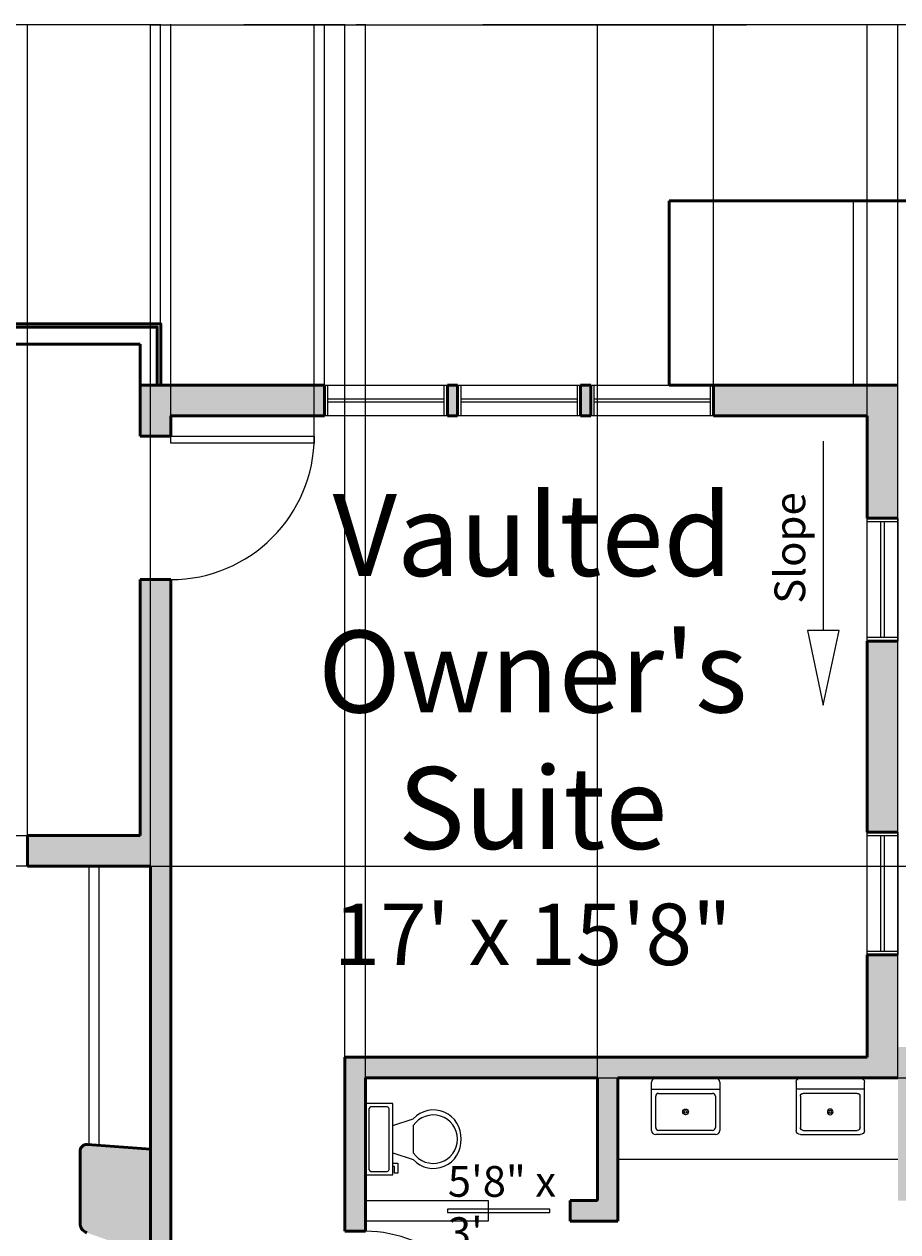
# Model space of a CAD drawing. Units: inches. Extents: x 296 to 2116, y 330 to 1460.
# Tile 5 of 9: x 752 to 1008, y 1106 to 1460. Entities that reach past the tile are written whole.
import ezdxf

# ---------------------------------------------------------------- set-up
doc = ezdxf.new("R2010")
doc.units = ezdxf.units.IN
for name, color, linetype, lineweight in [('A-ANNO-DIMS', 2, 'Continuous', 18), ('A-ANNO-SYMB', 2, 'Continuous', 18), ('A-ANNO-TEXT', 7, 'Continuous', 18), ('A-AREA-IDEN', 7, 'Continuous', 25), ('A-DOOR', 3, 'Continuous', 25), ('A-FLOR-FIXT', 8, 'Continuous', 18), ('A-FLOR-STRS', 40, 'Continuous', 25), ('A-GLAZ', 4, 'Continuous', 25), ('A-WALL', 7, 'Continuous', 50), ('A-WALL-PATT', 8, 'Continuous', 13)]:
    doc.layers.add(name, color=color, linetype=linetype, lineweight=lineweight)
doc.styles.add('ATTR', font='romans.shx', dxfattribs={"width": 0.8, "height": 1.075})
doc.styles.get("Standard").update_dxf_attribs({"font": 'arial.ttf'})
doc.dimstyles.get("Standard").update_dxf_attribs({"dimtxt": 0.18, "dimasz": 0.18, "dimexe": 0.18, "dimexo": 0.0625, "dimgap": 0.09, "dimtad": 0, "dimtih": 1, "dimtoh": 1, "dimdec": 4, "dimzin": 0, "dimdsep": 46, "dimtxsty": 'Standard', "dimcen": 0.09, "dimadec": 0, "dimazin": 0, "dimtfac": 1, "dimtdec": 4, "dimtofl": 0, "dimtmove": 0, "dimatfit": 3, "dimfxl": 1, "dimtolj": 1, "dimtzin": 0, "dimarcsym": 0})

# ---------------------------------------------------------------- blocks, each defined once
blk = doc.blocks.new('*U16')
for p, q in [((0, 0), (0, 4)), ((36, 0), (36, 4))]:
    blk.add_line(p, q)
blk.add_lwpolyline([(0, 0), (25.46, -25.46), (26.69, -24.22), (1.24, 1.24)], close=True)
blk.add_arc((0, 0), 36, 315, 0)
blk = doc.blocks.new('*U27')
for p, q in [((-36, 0), (-36, 4)), ((0, 0), (0, 4))]:
    blk.add_line(p, q)
blk.add_lwpolyline([(0, 0), (0, -36), (-1.75, -36), (-1.75, 0)], close=True)
blk.add_arc((0, 0), 36, 180, 270)
blk = doc.blocks.new('*U29')
for p, q in [((9.5, -6), (9.5, -2)), ((-10, -8.5), (-8, -8.5)), ((-10, -9.5), (-10, -8.5)), ((-7, -9.5), (-10, -9.5)), ((-8, -8.5), (-8, -8)), ((-7, -8), (-7, -9.5)), ((-4, -8), (-6, -14)), ((4, -8), (6, -14)), ((4, -14), (-4, -14))]:
    blk.add_line(p, q)
blk.add_lwpolyline([(10.5, -8), (10.5, 0), (-10.5, 0), (-10.5, -8)], close=True)
for points in [[(-9.5, -2), (-9.5, -6)], [(8.5, -1), (-8.5, -1)], [(-8.5, -7), (8.5, -7)]]:
    blk.add_lwpolyline(points)
for centre, radius, start, end in [((-8.625, -1.875), 0.8839, 81.8699, 188.1301), ((8.625, -1.875), 0.8839, 351.8699, 98.1301), ((-8.625, -6.125), 0.8839, 171.869898, 278.1301), ((8.625, -6.125), 0.8839, 261.8699, 8.1301), ((-0.4772, -19.9188), 8.0953, 133.01722, 273.38), ((0.0374, -19.8731), 7.127, 124.50543, 269.7), ((-0.0373, -19.8731), 7.127, 270.3, 55.4946), ((0.4773, -19.9188), 8.0953, 266.62, 46.9828)]:
    blk.add_arc(centre, radius, start, end)
blk = doc.blocks.new("24'' Sink Single PV")
blk.add_line((-12.00001, -3.999996), (12, -3.999996))
for points in [[(-10.5, 0), (10.5, 0)], [(-12.00001, -18.499996), (-12.00001, -1.5)], [(12, -1.5), (12, -18.499996)], [(-10.5, -17.499996), (-10.5, -6.499996)], [(-9.5, -5.499996), (9.5, -5.499996)], [(10.5, -6.499996), (10.5, -17.499996)], [(10.5, -19.999996), (-10.5, -19.999996)], [(9.5, -18.499996), (-9.5, -18.499996)]]:
    blk.add_lwpolyline(points)
for radius in [1, 0.5]:
    blk.add_circle((0, -11.999996), radius)
for centre, radius, start, end in [((-10.5, -1.5), 1.5, 90, 180), ((10.5, -1.5), 1.5, 0, 90), ((-9.5, -6.499996), 1, 90, 180), ((9.5, -6.499996), 1, 0, 90), ((-10.5, -18.499996), 1.5, 180, 270), ((-9.5, -17.499996), 1, 180, 270), ((9.5, -17.499996), 1, 270, 0), ((10.5, -18.499996), 1.5, 270, 0)]:
    blk.add_arc(centre, radius, start, end)
at = {"style": 'ATTR', "width": 0.8, "flags": 9}
blk.add_attdef('ESTCODE', (0, 0), '', height=0.0048, dxfattribs=at)
blk = doc.blocks.new('SLOPE-ARROW')
blk.add_line((739.99, 662.71), (684.54, 662.71))
blk.add_lwpolyline([(662.67, 662.71), (684.54, 658.1), (684.54, 667.32)], close=True)
blk = doc.blocks.new('*D45')
at = {"layer": 'A-ANNO-DIMS', "color": 0, "lineweight": -2, "transparency": 16777216}
for p, q in [((1156.58, 1407.95), (1235.3, 1407.95)), ((1235.12, 1407.77), (1235.12, 895.66)), ((1235.12, 383.18), (1235.12, 895.29)), ((609.63, 383), (1235.3, 383))]:
    blk.add_line(p, q, dxfattribs=at)
at = {"layer": 'A-ANNO-DIMS', "color": 0, "transparency": 16777216}
for points in [[(1235.09, 1407.77), (1235.15, 1407.77), (1235.12, 1407.95)], [(1235.09, 383.18), (1235.15, 383.18), (1235.12, 383)]]:
    blk.add_solid(points, dxfattribs=at)
at = {"layer": 'Defpoints', "color": 0, "transparency": 16777216}
for p in [(1156.52, 1407.95), (1235.12, 1407.95), (609.57, 383)]:
    blk.add_point(p, dxfattribs=at)
at = {"layer": 'A-ANNO-DIMS', "color": 0, "transparency": 16777216, "insert": (1235.12, 895.48), "char_height": 0.18, "attachment_point": 5}
blk.add_mtext('\\A1;1025', dxfattribs=at)
blk = doc.blocks.new('*D46')
at = {"layer": 'A-ANNO-DIMS', "color": 0, "lineweight": -2, "transparency": 16777216}
for p, q in [((399.52, 1371.02), (399.52, 1459.73)), ((399.7, 1459.55), (595.23, 1459.55)), ((791.34, 1459.55), (595.81, 1459.55)), ((791.52, 1372.02), (791.52, 1459.73))]:
    blk.add_line(p, q, dxfattribs=at)
at = {"layer": 'A-ANNO-DIMS', "color": 0, "transparency": 16777216}
for points in [[(399.7, 1459.58), (399.7, 1459.52), (399.52, 1459.55)], [(791.34, 1459.58), (791.34, 1459.52), (791.52, 1459.55)]]:
    blk.add_solid(points, dxfattribs=at)
at = {"layer": 'Defpoints', "color": 0, "transparency": 16777216}
for p in [(791.52, 1459.55), (399.52, 1370.95), (791.52, 1371.95)]:
    blk.add_point(p, dxfattribs=at)
at = {"layer": 'A-ANNO-DIMS', "color": 0, "transparency": 16777216, "insert": (595.52, 1459.55), "char_height": 0.18, "attachment_point": 5}
blk.add_mtext('\\A1;392', dxfattribs=at)
blk = doc.blocks.new('*D47')
at = {"layer": 'A-ANNO-DIMS', "color": 0, "lineweight": -2, "transparency": 16777216}
for p, q in [((791.52, 1372.02), (791.52, 1459.73)), ((791.7, 1459.55), (946.75, 1459.55)), ((1102.34, 1459.55), (947.29, 1459.55)), ((1102.52, 1354.02), (1102.52, 1459.73))]:
    blk.add_line(p, q, dxfattribs=at)
at = {"layer": 'A-ANNO-DIMS', "color": 0, "transparency": 16777216}
for points in [[(791.7, 1459.58), (791.7, 1459.52), (791.52, 1459.55)], [(1102.34, 1459.58), (1102.34, 1459.52), (1102.52, 1459.55)]]:
    blk.add_solid(points, dxfattribs=at)
at = {"layer": 'Defpoints', "color": 0, "transparency": 16777216}
for p in [(1102.52, 1459.55), (791.52, 1371.95), (1102.52, 1353.95)]:
    blk.add_point(p, dxfattribs=at)
at = {"layer": 'A-ANNO-DIMS', "color": 0, "transparency": 16777216, "insert": (947.02, 1459.55), "char_height": 0.18, "attachment_point": 5}
blk.add_mtext('\\A1;311', dxfattribs=at)
blk = doc.blocks.new('*D77')
at = {"layer": 'A-ANNO-DIMS', "color": 0, "lineweight": -2, "transparency": 16777216}
for p, q in [((845.52, 1157.02), (845.52, 1459.73)), ((845.7, 1459.55), (848.2, 1459.55)), ((851.34, 1459.55), (848.85, 1459.55)), ((851.52, 1151.02), (851.52, 1459.73))]:
    blk.add_line(p, q, dxfattribs=at)
at = {"layer": 'A-ANNO-DIMS', "color": 0, "transparency": 16777216}
for points in [[(845.7, 1459.58), (845.7, 1459.52), (845.52, 1459.55)], [(851.34, 1459.58), (851.34, 1459.52), (851.52, 1459.55)]]:
    blk.add_solid(points, dxfattribs=at)
at = {"layer": 'Defpoints', "color": 0, "transparency": 16777216}
for p in [(851.52, 1459.55), (845.52, 1156.95), (851.52, 1150.95)]:
    blk.add_point(p, dxfattribs=at)
at = {"layer": 'A-ANNO-DIMS', "color": 0, "transparency": 16777216, "insert": (848.52, 1459.55), "char_height": 0.18, "attachment_point": 5}
blk.add_mtext('\\A1;6.00', dxfattribs=at)
blk = doc.blocks.new('*D78')
at = {"layer": 'A-ANNO-DIMS', "color": 0, "lineweight": -2, "transparency": 16777216}
for p, q in [((398.52, 1192.06), (398.52, 1459.73)), ((398.7, 1459.55), (593.06, 1459.55)), ((788.34, 1459.55), (593.99, 1459.55)), ((788.52, 1213.06), (788.52, 1459.73))]:
    blk.add_line(p, q, dxfattribs=at)
at = {"layer": 'A-ANNO-DIMS', "color": 0, "transparency": 16777216}
for points in [[(398.7, 1459.58), (398.7, 1459.52), (398.52, 1459.55)], [(788.34, 1459.58), (788.34, 1459.52), (788.52, 1459.55)]]:
    blk.add_solid(points, dxfattribs=at)
at = {"layer": 'Defpoints', "color": 0, "transparency": 16777216}
for p in [(788.52, 1459.55), (788.52, 1213), (398.52, 1192)]:
    blk.add_point(p, dxfattribs=at)
at = {"layer": 'A-ANNO-DIMS', "color": 0, "transparency": 16777216, "insert": (593.52, 1459.55), "char_height": 0.18, "attachment_point": 5}
blk.add_mtext('\\A1;390.00', dxfattribs=at)
blk = doc.blocks.new('*D79')
at = {"layer": 'A-ANNO-DIMS', "color": 0, "lineweight": -2, "transparency": 16777216}
for p, q in [((788.522265, 1213.061588), (788.522265, 1459.734098)), ((788.702265, 1459.554098), (816.628868, 1459.554098)), ((845.342265, 1459.554098), (817.415662, 1459.554098)), ((845.522265, 1157.016598), (845.522265, 1459.734098))]:
    blk.add_line(p, q, dxfattribs=at)
at = {"layer": 'A-ANNO-DIMS', "color": 0, "transparency": 16777216}
for points in [[(788.702265, 1459.584098), (788.702265, 1459.524098), (788.522265, 1459.554098)], [(845.342265, 1459.584098), (845.342265, 1459.524098), (845.522265, 1459.554098)]]:
    blk.add_solid(points, dxfattribs=at)
at = {"layer": 'Defpoints', "color": 0, "transparency": 16777216}
for p in [(845.522265, 1459.554098), (788.522265, 1212.999088), (845.522265, 1156.954098)]:
    blk.add_point(p, dxfattribs=at)
at = {"layer": 'A-ANNO-DIMS', "color": 0, "transparency": 16777216, "insert": (817.022265, 1459.554098), "char_height": 0.18, "attachment_point": 5}
blk.add_mtext('\\A1;57.00', dxfattribs=at)
blk = doc.blocks.new('*D80')
at = {"layer": 'A-ANNO-DIMS', "color": 0, "lineweight": -2, "transparency": 16777216}
for p, q in [((851.52, 1151.02), (851.52, 1459.73)), ((851.7, 1459.55), (885.13, 1459.55)), ((919.34, 1459.55), (885.92, 1459.55)), ((919.52, 1115.02), (919.52, 1459.73))]:
    blk.add_line(p, q, dxfattribs=at)
at = {"layer": 'A-ANNO-DIMS', "color": 0, "transparency": 16777216}
for points in [[(851.7, 1459.58), (851.7, 1459.52), (851.52, 1459.55)], [(919.34, 1459.58), (919.34, 1459.52), (919.52, 1459.55)]]:
    blk.add_solid(points, dxfattribs=at)
at = {"layer": 'Defpoints', "color": 0, "transparency": 16777216}
for p in [(919.52, 1459.55), (851.52, 1150.95), (919.52, 1114.95)]:
    blk.add_point(p, dxfattribs=at)
at = {"layer": 'A-ANNO-DIMS', "color": 0, "transparency": 16777216, "insert": (885.52, 1459.55), "char_height": 0.18, "attachment_point": 5}
blk.add_mtext('\\A1;68.00', dxfattribs=at)
blk = doc.blocks.new('*D81')
at = {"layer": 'A-ANNO-DIMS', "color": 0, "lineweight": -2, "transparency": 16777216}
for p, q in [((919.52, 1115.02), (919.52, 1459.73)), ((919.7, 1459.55), (963.13, 1459.55)), ((1007.34, 1459.55), (963.92, 1459.55)), ((1007.52, 1151.02), (1007.52, 1459.73))]:
    blk.add_line(p, q, dxfattribs=at)
at = {"layer": 'A-ANNO-DIMS', "color": 0, "transparency": 16777216}
for points in [[(919.7, 1459.58), (919.7, 1459.52), (919.52, 1459.55)], [(1007.34, 1459.58), (1007.34, 1459.52), (1007.52, 1459.55)]]:
    blk.add_solid(points, dxfattribs=at)
at = {"layer": 'Defpoints', "color": 0, "transparency": 16777216}
for p in [(1007.52, 1459.55), (1007.52, 1150.95), (919.52, 1114.95)]:
    blk.add_point(p, dxfattribs=at)
at = {"layer": 'A-ANNO-DIMS', "color": 0, "transparency": 16777216, "insert": (963.52, 1459.55), "char_height": 0.18, "attachment_point": 5}
blk.add_mtext('\\A1;88.00', dxfattribs=at)
blk = doc.blocks.new('*D82')
at = {"layer": 'A-ANNO-DIMS', "color": 0, "lineweight": -2, "transparency": 16777216}
for p, q in [((794.52, 1345.02), (794.52, 1459.73)), ((794.7, 1459.55), (896.06, 1459.55)), ((998.34, 1459.55), (896.99, 1459.55)), ((998.52, 1345.02), (998.52, 1459.73))]:
    blk.add_line(p, q, dxfattribs=at)
at = {"layer": 'A-ANNO-DIMS', "color": 0, "transparency": 16777216}
for points in [[(794.7, 1459.58), (794.7, 1459.52), (794.52, 1459.55)], [(998.34, 1459.58), (998.34, 1459.52), (998.52, 1459.55)]]:
    blk.add_solid(points, dxfattribs=at)
at = {"layer": 'Defpoints', "color": 0, "transparency": 16777216}
for p in [(998.52, 1459.55), (794.52, 1344.95), (998.52, 1344.95)]:
    blk.add_point(p, dxfattribs=at)
at = {"layer": 'A-ANNO-DIMS', "color": 0, "transparency": 16777216, "insert": (896.52, 1459.55), "char_height": 0.18, "attachment_point": 5}
blk.add_mtext('\\A1;204.00', dxfattribs=at)
blk = doc.blocks.new('*D83')
at = {"layer": 'A-ANNO-DIMS', "color": 0, "lineweight": -2, "transparency": 16777216}
for p, q in [((851.58, 1150.95), (1235.3, 1150.95)), ((1235.12, 1150.77), (1235.12, 1109.14)), ((1235.12, 1067.13), (1235.12, 1108.77)), ((851.58, 1066.95), (1235.3, 1066.95))]:
    blk.add_line(p, q, dxfattribs=at)
at = {"layer": 'A-ANNO-DIMS', "color": 0, "transparency": 16777216}
for points in [[(1235.09, 1150.77), (1235.15, 1150.77), (1235.12, 1150.95)], [(1235.09, 1067.13), (1235.15, 1067.13), (1235.12, 1066.95)]]:
    blk.add_solid(points, dxfattribs=at)
at = {"layer": 'Defpoints', "color": 0, "transparency": 16777216}
for p in [(851.52, 1150.95), (1235.12, 1150.95), (851.52, 1066.95)]:
    blk.add_point(p, dxfattribs=at)
at = {"layer": 'A-ANNO-DIMS', "color": 0, "transparency": 16777216, "insert": (1235.12, 1108.95), "char_height": 0.18, "attachment_point": 5}
blk.add_mtext('\\A1;84.00', dxfattribs=at)
blk = doc.blocks.new('*D85')
at = {"layer": 'A-ANNO-DIMS', "color": 0, "lineweight": -2, "transparency": 16777216}
for p, q in [((788.58, 1213), (1235.3, 1213)), ((1235.12, 1212.82), (1235.12, 1075.18)), ((1235.12, 937.18), (1235.12, 1074.82)), ((788.58, 937), (1235.3, 937))]:
    blk.add_line(p, q, dxfattribs=at)
at = {"layer": 'A-ANNO-DIMS', "color": 0, "transparency": 16777216}
for points in [[(1235.09, 1212.82), (1235.15, 1212.82), (1235.12, 1213)], [(1235.09, 937.18), (1235.15, 937.18), (1235.12, 937)]]:
    blk.add_solid(points, dxfattribs=at)
at = {"layer": 'Defpoints', "color": 0, "transparency": 16777216}
for p in [(788.52, 1213), (1235.12, 1213), (788.52, 937)]:
    blk.add_point(p, dxfattribs=at)
at = {"layer": 'A-ANNO-DIMS', "color": 0, "transparency": 16777216, "insert": (1235.12, 1075), "char_height": 0.18, "attachment_point": 5}
blk.add_mtext('\\A1;276.00', dxfattribs=at)
blk = doc.blocks.new('*D100')
at = {"layer": 'A-ANNO-DIMS', "color": 0, "lineweight": -2, "transparency": 16777216}
for p, q in [((794.52, 1339.02), (794.52, 1459.73)), ((794.7, 1459.55), (815.13, 1459.55)), ((836.34, 1459.55), (815.92, 1459.55)), ((836.52, 1339.02), (836.52, 1459.73))]:
    blk.add_line(p, q, dxfattribs=at)
at = {"layer": 'A-ANNO-DIMS', "color": 0, "transparency": 16777216}
for points in [[(794.7, 1459.58), (794.7, 1459.52), (794.52, 1459.55)], [(836.34, 1459.58), (836.34, 1459.52), (836.52, 1459.55)]]:
    blk.add_solid(points, dxfattribs=at)
at = {"layer": 'Defpoints', "color": 0, "transparency": 16777216}
for p in [(836.52, 1459.55), (794.52, 1338.95), (836.52, 1338.95)]:
    blk.add_point(p, dxfattribs=at)
at = {"layer": 'A-ANNO-DIMS', "color": 0, "transparency": 16777216, "insert": (815.52, 1459.55), "char_height": 0.18, "attachment_point": 5}
blk.add_mtext('\\A1;42.00', dxfattribs=at)
blk = doc.blocks.new('*D104')
at = {"layer": 'A-ANNO-DIMS', "color": 0, "lineweight": -2, "transparency": 16777216}
for p, q in [((612.52, 1222.06), (612.52, 1459.73)), ((612.7, 1459.55), (682.07, 1459.55)), ((752.34, 1459.55), (682.98, 1459.55)), ((752.52, 1222.06), (752.52, 1459.73))]:
    blk.add_line(p, q, dxfattribs=at)
at = {"layer": 'A-ANNO-DIMS', "color": 0, "transparency": 16777216}
for points in [[(612.7, 1459.58), (612.7, 1459.52), (612.52, 1459.55)], [(752.34, 1459.58), (752.34, 1459.52), (752.52, 1459.55)]]:
    blk.add_solid(points, dxfattribs=at)
at = {"layer": 'Defpoints', "color": 0, "transparency": 16777216}
for p in [(752.52, 1459.55), (612.52, 1222), (752.52, 1222)]:
    blk.add_point(p, dxfattribs=at)
at = {"layer": 'A-ANNO-DIMS', "color": 0, "transparency": 16777216, "insert": (682.52, 1459.55), "char_height": 0.18, "attachment_point": 5}
blk.add_mtext('\\A1;140.00', dxfattribs=at)
blk = doc.blocks.new('*D106')
at = {"layer": 'A-ANNO-DIMS', "color": 0, "lineweight": -2, "transparency": 16777216}
for p, q in [((839.52, 1354.02), (839.52, 1459.73)), ((839.7, 1459.55), (896.07, 1459.55)), ((953.34, 1459.55), (896.98, 1459.55)), ((953.52, 1354.02), (953.52, 1459.73))]:
    blk.add_line(p, q, dxfattribs=at)
at = {"layer": 'A-ANNO-DIMS', "color": 0, "transparency": 16777216}
for points in [[(839.7, 1459.58), (839.7, 1459.52), (839.52, 1459.55)], [(953.34, 1459.58), (953.34, 1459.52), (953.52, 1459.55)]]:
    blk.add_solid(points, dxfattribs=at)
at = {"layer": 'Defpoints', "color": 0, "transparency": 16777216}
for p in [(953.52, 1459.55), (839.52, 1353.95), (953.52, 1353.95)]:
    blk.add_point(p, dxfattribs=at)
at = {"layer": 'A-ANNO-DIMS', "color": 0, "transparency": 16777216, "insert": (896.52, 1459.55), "char_height": 0.18, "attachment_point": 5}
blk.add_mtext('\\A1;114.00', dxfattribs=at)

msp = doc.modelspace()

# ---------------------------------------------------------------- hatches: boundary and pattern name
at = {"layer": 'A-WALL-PATT'}
h = msp.add_hatch(color=256, dxfattribs=at)
h.dxf.hatch_style = 1
h.paths.add_polyline_path([(656.5723, 927.9991), (668.5723, 927.9991), (668.5723, 936.9991), (650.5723, 936.9991), (650.5723, 897.9991), (356.5223, 897.9991), (356.5223, 955.9991), (347.5223, 955.9991), (347.5223, 888.9991), (423.5723, 888.9991), (423.5723, 766.9991), (432.5723, 766.9991), (432.5723, 834.9991), (453.5723, 834.9991), (468.5723, 834.9991), (468.5723, 840.9991), (432.5723, 840.9991), (432.5723, 888.9991), (504.5723, 888.9991), (504.5723, 840.9991), (504.5723, 834.9991), (531.6223, 834.9991), (531.6223, 768.5344), (527.8443, 764.7564), (530.6728, 761.928), (532.087, 760.5138), (540.5723, 768.9991), (598.0723, 768.9991), (598.0723, 777.9991), (601.8223, 777.9991), (601.8223, 782.1991), (601.8223, 783.9991), (598.0723, 783.9991), (598.0723, 798.9991), (592.0723, 798.9991), (592.0723, 774.9991), (537.6223, 774.9991), (537.6223, 834.9991), (592.0723, 834.9991), (592.0723, 828.9991), (598.0723, 828.9991), (598.0723, 834.9991), (647.5723, 834.9991), (647.5723, 828.9991), (656.5723, 828.9991), (656.5723, 846.9991), (650.5723, 846.9991), (647.5723, 846.9991), (647.5723, 840.9991), (510.5723, 840.9991), (510.5723, 888.9991), (647.5723, 888.9991), (647.5723, 882.9991), (656.5723, 882.9991)])
h.paths.add_polyline_path([(432.5723, 730.9991), (496.5723, 730.9991), (496.5723, 724.9991), (502.5723, 724.9991), (502.5723, 730.9991), (506.6311, 735.058), (502.3885, 739.3006), (500.087, 736.9991), (432.5723, 736.9991), (432.5723, 742.9991), (423.5723, 742.9991), (423.5723, 641.9991), (490.5723, 641.9991), (490.5723, 597.9991), (531.5723, 597.9991), (531.5723, 606.9991), (499.5723, 606.9991), (499.5723, 650.9991), (502.5723, 650.9991), (502.5723, 659.9991), (496.5723, 659.9991), (493.5723, 659.9991), (493.5723, 650.9991), (432.5723, 650.9991)])
h.paths.add_polyline_path([(656.5723, 689.4991), (662.5473, 689.4991), (662.5473, 698.4991), (656.5723, 698.4991), (656.5723, 789.9991), (647.5723, 789.9991), (647.5723, 783.9991), (643.8223, 783.9991), (643.8223, 777.9991), (647.5723, 777.9991), (647.5723, 606.9991), (615.5723, 606.9991), (615.5723, 597.9991), (656.5723, 597.9991)])
h.paths.add_polyline_path([(761.5223, 780.9541), (797.5223, 780.9541), (797.5223, 789.9541), (761.5223, 789.9541), (761.5223, 858.9541), (797.5223, 858.9541), (797.5223, 867.9541), (752.5223, 867.9541), (752.5223, 698.4991), (746.5473, 698.4991), (746.5473, 694.2991), (746.5473, 689.4991), (752.5223, 689.4991), (752.5223, 624.9541), (761.5223, 624.9541)])
h.paths.add_polyline_path([(1102.5223, 795.9541), (1093.5223, 795.9541), (1093.5223, 789.9541), (1063.5223, 789.9541), (881.5223, 789.9541), (881.5223, 837.9541), (911.5223, 837.9541), (911.5223, 849.9541), (907.5223, 849.9541), (905.5223, 849.9541), (905.5223, 843.9541), (845.5223, 843.9541), (845.5223, 834.9541), (849.0223, 834.9541), (851.5223, 834.9541), (851.5223, 837.9541), (875.5223, 837.9541), (875.5223, 789.9541), (851.5223, 789.9541), (851.5223, 792.9541), (845.5223, 792.9541), (845.5223, 789.9541), (833.5223, 789.9541), (833.5223, 785.1541), (833.5223, 780.9541), (1049.5223, 780.9541), (1049.5223, 726.9541), (1053.7223, 726.9541), (1058.5223, 726.9541), (1058.5223, 780.9541), (1102.5223, 780.9541)])
h.paths.add_polyline_path([(761.5223, 588.9541), (752.5223, 588.9541), (752.5223, 564.9541), (761.5223, 564.9541)])
h.paths.add_polyline_path([(809.5223, 480.9541), (761.5223, 480.9541), (761.5223, 528.9541), (752.5223, 528.9541), (752.5223, 471.9541), (809.5223, 471.9541)])
h.paths.add_polyline_path([(1058.5223, 684.9541), (1049.5223, 684.9541), (1049.5223, 480.9541), (1001.5223, 480.9541), (1001.5223, 476.4541), (1001.5223, 471.9541), (1058.5223, 471.9541)])
h.paths.add_polyline_path([(794.5223, 1013.9991), (800.5223, 1013.9991), (800.5223, 1019.9991), (794.5223, 1019.9991), (794.5223, 1296.9541), (785.5223, 1296.9541), (785.5223, 1221.9991), (752.5223, 1221.9991), (752.5223, 1212.9991), (788.5223, 1212.9991), (788.5223, 936.9991), (752.5223, 936.9991), (752.5223, 927.9991), (794.5223, 927.9991)])
h.paths.add_polyline_path([(450.0223, 1191.9991), (398.5223, 1191.9991), (398.5223, 1137.9991), (407.5223, 1137.9991), (407.5223, 1182.9991), (450.0223, 1182.9991)])
h.paths.add_polyline_path([(576.5223, 1212.9991), (612.5223, 1212.9991), (612.5223, 1221.9991), (567.5223, 1221.9991), (567.5223, 1191.9991), (540.0223, 1191.9991), (540.0223, 1182.9991), (576.5223, 1182.9991)])
h.paths.add_polyline_path([(407.5223, 1060.9991), (398.5223, 1060.9991), (398.5223, 1030.9991), (392.5223, 1030.9991), (392.5223, 1021.9991), (407.5223, 1021.9991)])
h.paths.add_polyline_path([(356.5223, 1030.9991), (347.5223, 1030.9991), (347.5223, 1015.9991), (356.5223, 1015.9991), (356.5223, 1021.9991)])
h.paths.add_polyline_path([(788.5223, 1129.9991), (770.0334, 1131.3572, 0.43585667), (767.8869, 1129.3626), (767.8869, 1108.3618, 0.31855172), (769.8942, 1105.5308), (788.5223, 1098.9991)], flags=17)
h.paths.add_polyline_path([(788.5223, 1050.9991), (769.8942, 1044.4674, 0.31855172), (767.8869, 1041.6364), (767.8869, 1020.6356, 0.43585667), (770.0334, 1018.641), (788.5223, 1019.9991)], flags=17)
h.paths.add_polyline_path([(893.5223, 1066.9541), (851.5223, 1066.9541), (851.5223, 1069.9541), (845.5223, 1069.9541), (845.5223, 1019.9991), (839.5223, 1019.9991), (839.5223, 1013.9991), (845.5223, 1013.9991), (845.5223, 891.9541), (863.5223, 891.9541), (863.5223, 897.9541), (851.5223, 897.9541), (851.5223, 927.9541), (905.5223, 927.9541), (905.5223, 897.9541), (893.5223, 897.9541), (893.5223, 891.9541), (905.5223, 891.9541), (905.5223, 885.9541), (911.5223, 885.9541), (911.5223, 927.9541), (1030.5223, 927.9541), (1030.5223, 936.9541), (1013.5223, 936.9541), (1013.5223, 996.9541), (1093.5223, 996.9541), (1093.5223, 936.9541), (1066.5223, 936.9541), (1066.5223, 927.9541), (1093.5223, 927.9541), (1093.5223, 921.9541), (1102.5223, 921.9541), (1102.5223, 1013.9541), (1093.5223, 1013.9541), (1093.5223, 1002.9541), (1013.5223, 1002.9541), (1013.5223, 1060.9541), (1013.5223, 1066.9541), (1007.5223, 1066.9541), (1007.5223, 1042.9541), (977.5223, 1042.9541), (977.5223, 1066.9541), (965.5223, 1066.9541), (965.5223, 1060.9541), (971.5223, 1060.9541), (971.5223, 1036.9541), (1007.5223, 1036.9541), (1007.5223, 936.9541), (851.5223, 936.9541), (851.5223, 1060.9541), (893.5223, 1060.9541)])
h.paths.add_polyline_path([(851.5223, 1150.9541), (919.5223, 1150.9541), (919.5223, 1114.9541), (911.5223, 1114.9541), (911.5223, 1108.9541), (925.5223, 1108.9541), (925.5223, 1150.9541), (1007.5223, 1150.9541), (1007.5223, 1114.9541), (1013.5223, 1114.9541), (1013.5223, 1150.9541), (1046.5223, 1150.9541), (1046.5223, 1159.9541), (1007.5223, 1159.9541), (1007.5223, 1186.9541), (998.5223, 1186.9541), (998.5223, 1156.9541), (845.5223, 1156.9541), (845.5223, 1105.9541), (851.5223, 1105.9541)])
h.paths.add_polyline_path([(1102.5223, 1156.9541), (1102.5223, 1159.9541), (1088.5223, 1159.9541), (1088.5223, 1150.9541), (1093.5223, 1150.9541), (1093.5223, 1147.9541), (1102.5223, 1147.9541)])
h.paths.add_polyline_path([(1102.5223, 1111.9541), (1093.5223, 1111.9541), (1093.5223, 1066.9541), (1047.5223, 1066.9541), (1047.5223, 1030.9541), (1053.5223, 1030.9541), (1053.5223, 1060.9541), (1093.5223, 1060.9541), (1093.5223, 1049.9541), (1102.5223, 1049.9541)])
h.paths.add_polyline_path([(1102.5223, 837.9541), (1093.5223, 837.9541), (1093.5223, 831.9541), (1102.5223, 831.9541)], flags=17)
h.paths.add_polyline_path([(1102.5223, 879.9541), (1093.5223, 879.9541), (1093.5223, 873.9541), (1102.5223, 873.9541)])
h.paths.add_polyline_path([(839.5223, 1353.9541), (785.5223, 1353.9541), (785.5223, 1338.9541), (794.5223, 1338.9541), (794.5223, 1344.9541), (839.5223, 1344.9541)])
h.paths.add_polyline_path([(1007.5223, 1353.9541), (953.5223, 1353.9541), (953.5223, 1344.9541), (998.5223, 1344.9541), (998.5223, 1314.9541), (1007.5223, 1314.9541)])
h.paths.add_polyline_path([(917.5223, 1353.9541), (914.5223, 1353.9541), (914.5223, 1344.9541), (917.5223, 1344.9541)])
h.paths.add_polyline_path([(878.5223, 1353.9541), (875.5223, 1353.9541), (875.5223, 1344.9541), (878.5223, 1344.9541)])
h.paths.add_polyline_path([(1007.5223, 1278.9541), (998.5223, 1278.9541), (998.5223, 1222.9541), (1007.5223, 1222.9541)])
h.paths.add_polyline_path([(407.5223, 1101.9991), (398.5223, 1101.9991), (398.5223, 1096.9991), (407.5223, 1096.9991)])
h.paths.add_polyline_path([(560.5723, 606.9991), (557.5723, 606.9991), (557.5723, 597.9991), (560.5723, 597.9991)])
h.paths.add_polyline_path([(589.5723, 606.9991), (586.5723, 606.9991), (586.5723, 597.9991), (589.5723, 597.9991)])

# ---------------------------------------------------------------- linework, layer by layer
at = {"layer": 'A-DOOR'}
for points in [[(752.5223, 1221.9991), (752.5223, 1212.9991), (612.5223, 1212.9991), (612.5223, 1221.9991)], [(851.5223, 1114.9541), (887.5223, 1114.9541), (887.5223, 1108.9541), (851.5223, 1108.9541)], [(875.5223, 1111.4541), (905.5223, 1111.4541), (905.5223, 1112.4541), (875.5223, 1112.4541)]]:
    msp.add_lwpolyline(points, close=True, dxfattribs=at)
at = {"layer": 'A-FLOR-FIXT'}
for p, q in [((770.5223, 1131.3213), (770.5223, 1212.9991)), ((773.5223, 1131.1009), (773.5223, 1212.9991)), ((1007.5223, 1126.9541), (925.5223, 1126.9541))]:
    msp.add_line(p, q, dxfattribs=at)
at = {"layer": 'A-FLOR-STRS'}
msp.add_line((994.5223, 1353.9541), (994.5223, 1407.9541), dxfattribs=at)
at = {"layer": 'A-GLAZ'}
for p, q in [((840.5223, 1344.9541), (840.5223, 1353.9541)), ((874.5223, 1353.9541), (874.5223, 1344.9541)), ((879.5223, 1344.9541), (879.5223, 1353.9541)), ((913.5223, 1353.9541), (913.5223, 1344.9541)), ((918.5223, 1344.9541), (918.5223, 1353.9541)), ((952.5223, 1353.9541), (952.5223, 1344.9541)), ((840.5223, 1349.9541), (874.5223, 1349.9541)), ((874.5223, 1348.9541), (840.5223, 1348.9541)), ((879.5223, 1349.9541), (913.5223, 1349.9541)), ((913.5223, 1348.9541), (879.5223, 1348.9541)), ((918.5223, 1349.9541), (952.5223, 1349.9541)), ((952.5223, 1348.9541), (918.5223, 1348.9541)), ((998.5223, 1313.9541), (1007.5223, 1313.9541)), ((1002.5223, 1279.9541), (1002.5223, 1313.9541)), ((1003.5223, 1313.9541), (1003.5223, 1279.9541)), ((1007.5223, 1279.9541), (998.5223, 1279.9541)), ((998.5223, 1221.9541), (1007.5223, 1221.9541)), ((1002.5223, 1187.9541), (1002.5223, 1221.9541)), ((1003.5223, 1221.9541), (1003.5223, 1187.9541)), ((1007.5223, 1187.9541), (998.5223, 1187.9541))]:
    msp.add_line(p, q, dxfattribs=at)
for points in [[(875.5223, 1353.9541), (875.5223, 1344.9541), (839.5223, 1344.9541), (839.5223, 1353.9541)], [(914.5223, 1353.9541), (914.5223, 1344.9541), (878.5223, 1344.9541), (878.5223, 1353.9541)], [(953.5223, 1353.9541), (953.5223, 1344.9541), (917.5223, 1344.9541), (917.5223, 1353.9541)], [(1007.5223, 1278.9541), (998.5223, 1278.9541), (998.5223, 1314.9541), (1007.5223, 1314.9541)], [(1007.5223, 1186.9541), (998.5223, 1186.9541), (998.5223, 1222.9541), (1007.5223, 1222.9541)]]:
    msp.add_lwpolyline(points, close=True, dxfattribs=at)
at = {"layer": 'A-WALL'}
for p, q in [((940.5223, 1353.9541), (940.5223, 1407.9541)), ((940.5223, 1407.9541), (1156.5223, 1407.9541)), ((785.5223, 1365.9541), (404.5223, 1365.9541)), ((785.5223, 1353.9541), (785.5223, 1365.9541)), ((839.5223, 1353.9541), (785.5223, 1353.9541)), ((785.5223, 1338.9541), (785.5223, 1353.9541)), ((839.5223, 1344.9541), (839.5223, 1353.9541)), ((875.5223, 1344.9541), (875.5223, 1353.9541)), ((878.5223, 1353.9541), (875.5223, 1353.9541)), ((878.5223, 1344.9541), (878.5223, 1353.9541)), ((914.5223, 1344.9541), (914.5223, 1353.9541)), ((917.5223, 1353.9541), (914.5223, 1353.9541)), ((917.5223, 1344.9541), (917.5223, 1353.9541)), ((1007.5223, 1353.9541), (940.5223, 1353.9541)), ((953.5223, 1344.9541), (953.5223, 1353.9541)), ((839.5223, 1344.9541), (794.5223, 1344.9541)), ((794.5223, 1338.9541), (794.5223, 1344.9541)), ((878.5223, 1344.9541), (875.5223, 1344.9541)), ((917.5223, 1344.9541), (914.5223, 1344.9541)), ((998.5223, 1344.9541), (953.5223, 1344.9541)), ((998.5223, 1314.9541), (998.5223, 1344.9541)), ((794.5223, 1338.9541), (785.5223, 1338.9541)), ((998.5223, 1314.9541), (1007.5223, 1314.9541)), ((785.5223, 1221.9991), (785.5223, 1296.9541)), ((794.5223, 1296.9541), (785.5223, 1296.9541)), ((794.5223, 1019.9991), (794.5223, 1296.9541)), ((998.5223, 1278.9541), (1007.5223, 1278.9541)), ((998.5223, 1222.9541), (998.5223, 1278.9541)), ((785.5223, 1221.9991), (752.5223, 1221.9991)), ((752.5223, 1212.9991), (752.5223, 1221.9991)), ((998.5223, 1222.9541), (1007.5223, 1222.9541)), ((788.5223, 1212.9991), (752.5223, 1212.9991)), ((788.5223, 936.9991), (788.5223, 1212.9991)), ((998.5223, 1156.9541), (998.5223, 1186.9541)), ((998.5223, 1186.9541), (1007.5223, 1186.9541)), ((845.5223, 1105.9541), (845.5223, 1156.9541)), ((998.5223, 1156.9541), (845.5223, 1156.9541)), ((919.5223, 1150.9541), (851.5223, 1150.9541)), ((851.5223, 1105.9541), (851.5223, 1150.9541)), ((919.5223, 1114.9541), (919.5223, 1150.9541)), ((925.5223, 1108.9541), (925.5223, 1150.9541)), ((1007.5223, 1150.9541), (925.5223, 1150.9541)), ((767.8869, 1108.3618), (767.8869, 1129.3626)), ((788.5223, 1129.9991), (770.0334, 1131.3572)), ((919.5223, 1114.9541), (911.5223, 1114.9541)), ((911.5223, 1108.9541), (911.5223, 1114.9541)), ((925.5223, 1108.9541), (911.5223, 1108.9541)), ((851.5223, 1105.9541), (845.5223, 1105.9541))]:
    msp.add_line(p, q, dxfattribs=at)
for points in [[(791.5223, 1353.9541), (791.5223, 1371.9541), (398.5223, 1371.9541), (398.5223, 1191.9991)], [(790.5223, 1353.9541), (790.5223, 1370.9541), (399.5223, 1370.9541), (399.5223, 1191.9991)]]:
    msp.add_lwpolyline(points, dxfattribs=at)
for centre, radius, start, end in [((769.8869, 1129.3626), 2, 85.798796, 180), ((770.8869, 1108.3618), 3, 180, 250.67747)]:
    msp.add_arc(centre, radius, start, end, dxfattribs=at)

# ---------------------------------------------------------------- block references
at = {"layer": 'A-ANNO-SYMB', "rotation": 90}
msp.add_blockref('SLOPE-ARROW', (1648.3817, 597.4809), dxfattribs=at)
at = {"layer": 'A-DOOR', "xscale": 1.166666666666666, "yscale": 1.166666666666666, "zscale": 1.166666666666666, "rotation": 89.99999999999999}
msp.add_blockref('*U27', (794.5223, 1338.9541), dxfattribs=at)
at = {"layer": 'A-DOOR', "rotation": 90.00000000000003}
msp.add_blockref('*U16', (851.5223, 1069.9541), dxfattribs=at)
at = {"layer": 'A-FLOR-FIXT', "yscale": 0.8333413357028808, "zscale": 0.8333413357028808}
for p, xscale in [((945.3238, 1150.9541), 0.8333413357028808), ((987.7207, 1150.9541), -0.8333413357028808)]:
    msp.add_blockref("24'' Sink Single PV", p, dxfattribs=dict(at, xscale=xscale))
at = {"layer": 'A-FLOR-FIXT', "rotation": 90}
msp.add_blockref('*U29', (851.5223, 1132.9541), dxfattribs=at)

# ---------------------------------------------------------------- texts
at = {"layer": 'A-ANNO-TEXT', "insert": (971.3829, 1285.2149), "char_height": 9, "attachment_point": 1, "rotation": 90}
msp.add_mtext_dynamic_manual_height_columns('\\pxqc;Slope', width=41.969454, gutter_width=12.5, heights=[0], dxfattribs=at)
at = {"layer": 'A-AREA-IDEN', "attachment_point": 1}
for s, width, insert, char_height in [('\\pxqc;Vaulted\\P{\\fArial|b1|i0|c0|p34;Owner\'s Suite\\P\\fArial|b0|i0|c0|p34;\\H0.75x;17\' x 15\'8"}', 144.779934, (828.1335, 1322.0163), 24), ('5\'8" x 3\'', 42.589055, (875.6571, 1125.0707), 9)]:
    msp.add_mtext_dynamic_manual_height_columns(s, width=width, gutter_width=12.5, heights=[0], dxfattribs=dict(at, insert=insert, char_height=char_height))

# ---------------------------------------------------------------- dimensions: what is measured, and where the dimension line sits
at = {"layer": 'A-ANNO-DIMS'}
for base, p1, p2, override, picture, middle in [((788.5223, 1459.5541), (398.5223, 1191.9991), (788.5223, 1212.9991), {"dimdec": 2, "dimlfac": 1, "dimrnd": 0, "dimzin": 0, "dimdsep": 46, "dimlunit": 2}, '*D78', (593.5223, 1459.5541)), ((791.5223, 1459.5541), (399.5223, 1370.9541), (791.5223, 1371.9541), {"dimdec": 0, "dimlfac": 1, "dimrnd": 0, "dimzin": 0, "dimdsep": 46, "dimlunit": 2}, '*D46', (595.5223, 1459.5541)), ((752.5223, 1459.5541), (612.5223, 1221.9991), (752.5223, 1221.9991), {"dimdec": 2, "dimlfac": 1, "dimrnd": 0, "dimzin": 0, "dimdsep": 46, "dimlunit": 2}, '*D104', (682.5223, 1459.5541)), ((845.5223, 1459.5541), (788.5223, 1212.9991), (845.5223, 1156.9541), {"dimdec": 2, "dimlfac": 1, "dimrnd": 0, "dimzin": 0, "dimdsep": 46, "dimlunit": 2}, '*D79', (817.0223, 1459.5541)), ((1102.5223, 1459.5541), (791.5223, 1371.9541), (1102.5223, 1353.9541), {"dimdec": 0, "dimlfac": 1, "dimrnd": 0, "dimzin": 0, "dimdsep": 46, "dimlunit": 2}, '*D47', (947.0223, 1459.5541)), ((998.5223, 1459.5541), (794.5223, 1344.9541), (998.5223, 1344.9541), {"dimdec": 2, "dimlfac": 1, "dimrnd": 0, "dimzin": 0, "dimdsep": 46, "dimlunit": 2}, '*D82', (896.5223, 1459.5541)), ((836.5223, 1459.5541), (794.5223, 1338.9541), (836.5223, 1338.9541), {"dimdec": 2, "dimlfac": 1, "dimrnd": 0, "dimzin": 0, "dimdsep": 46, "dimlunit": 2}, '*D100', (815.5223, 1459.5541)), ((953.5223, 1459.5541), (839.5223, 1353.9541), (953.5223, 1353.9541), {"dimdec": 2, "dimlfac": 1, "dimrnd": 0, "dimzin": 0, "dimdsep": 46, "dimlunit": 2}, '*D106', (896.5223, 1459.5541)), ((851.5223, 1459.5541), (845.5223, 1156.9541), (851.5223, 1150.9541), {"dimdec": 2, "dimlfac": 1, "dimrnd": 0, "dimzin": 0, "dimdsep": 46, "dimlunit": 2}, '*D77', (848.5223, 1459.5541)), ((919.5223, 1459.5541), (851.5223, 1150.9541), (919.5223, 1114.9541), {"dimdec": 2, "dimlfac": 1, "dimrnd": 0, "dimzin": 0, "dimdsep": 46, "dimlunit": 2}, '*D80', (885.5223, 1459.5541)), ((1007.5223, 1459.5541), (919.5223, 1114.9541), (1007.5223, 1150.9541), {"dimdec": 2, "dimlfac": 1, "dimrnd": 0, "dimzin": 0, "dimdsep": 46, "dimlunit": 2}, '*D81', (963.5223, 1459.5541))]:
    dim = msp.add_linear_dim(base=base, p1=p1, p2=p2, dimstyle='Standard', override=override, dxfattribs=at)
    dim.commit()
    dim.dimension.update_dxf_attribs({"geometry": picture, "text_midpoint": middle})
for base, p1, p2, override, picture, middle in [((1235.1223, 1407.9541), (609.5723, 382.9991), (1156.5223, 1407.9541), {"dimdec": 0, "dimlfac": 1, "dimrnd": 0, "dimzin": 0, "dimdsep": 46, "dimlunit": 2}, '*D45', (1235.1223, 895.4766)), ((1235.1223, 1212.9991), (788.5223, 936.9991), (788.5223, 1212.9991), {"dimdec": 2, "dimlfac": 1, "dimrnd": 0, "dimzin": 0, "dimdsep": 46, "dimlunit": 2}, '*D85', (1235.1223, 1074.9991)), ((1235.1223, 1150.9541), (851.5223, 1066.9541), (851.5223, 1150.9541), {"dimdec": 2, "dimlfac": 1, "dimrnd": 0, "dimzin": 0, "dimdsep": 46, "dimlunit": 2}, '*D83', (1235.1223, 1108.9541))]:
    dim = msp.add_linear_dim(base=base, p1=p1, p2=p2, angle=90, dimstyle='Standard', override=override, dxfattribs=at)
    dim.commit()
    dim.dimension.update_dxf_attribs({"geometry": picture, "text_midpoint": middle})

doc.saveas('drawing.dxf')
